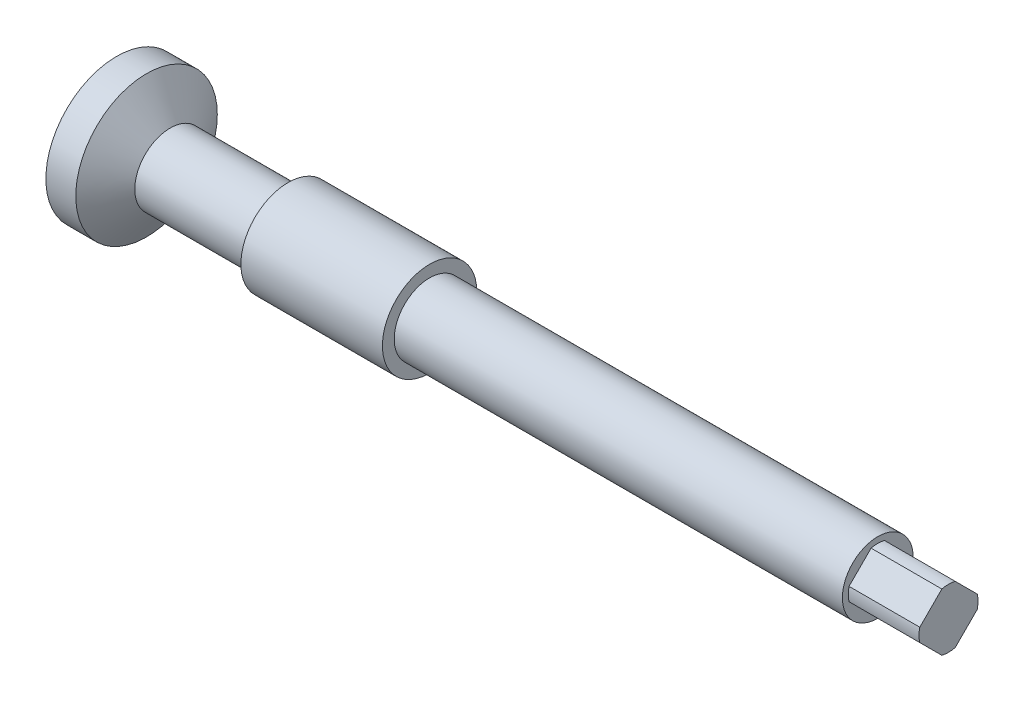
ISO-10303-21;
HEADER;
FILE_DESCRIPTION(('STEP AP214'),'2;1');
FILE_NAME('part.step','',(''),(''),'','','');
FILE_SCHEMA(('AUTOMOTIVE_DESIGN { 1 0 10303 214 1 1 1 1 }'));
ENDSEC;
DATA;
#1=APPLICATION_CONTEXT('core data for automotive mechanical design processes');
#2=APPLICATION_PROTOCOL_DEFINITION('international standard','automotive_design',2000,#1);
#3=PRODUCT_CONTEXT('',#1,'mechanical');
#4=PRODUCT('Part','Part','',(#3));
#5=PRODUCT_RELATED_PRODUCT_CATEGORY('part','',(#4));
#6=PRODUCT_DEFINITION_FORMATION('','',#4);
#7=PRODUCT_DEFINITION_CONTEXT('part definition',#1,'design');
#8=PRODUCT_DEFINITION('design','',#6,#7);
#9=PRODUCT_DEFINITION_SHAPE('','',#8);
#10=(LENGTH_UNIT() NAMED_UNIT(*) SI_UNIT(.MILLI.,.METRE.));
#11=(NAMED_UNIT(*) PLANE_ANGLE_UNIT() SI_UNIT($,.RADIAN.));
#12=(NAMED_UNIT(*) SI_UNIT($,.STERADIAN.) SOLID_ANGLE_UNIT());
#13=UNCERTAINTY_MEASURE_WITH_UNIT(LENGTH_MEASURE(1.E-05),#10,'distance_accuracy_value','');
#14=(GEOMETRIC_REPRESENTATION_CONTEXT(3) GLOBAL_UNCERTAINTY_ASSIGNED_CONTEXT((#13)) GLOBAL_UNIT_ASSIGNED_CONTEXT((#10,
#11,#12)) REPRESENTATION_CONTEXT('',''));
#15=CARTESIAN_POINT('',(0.,0.,0.));
#16=DIRECTION('',(0.,0.,1.));
#17=DIRECTION('',(1.,0.,0.));
#18=AXIS2_PLACEMENT_3D('',#15,#16,#17);
#19=CARTESIAN_POINT('',(0.,0.,0.));
#20=DIRECTION('',(1.,0.,0.));
#21=DIRECTION('',(0.,0.,-1.));
#22=AXIS2_PLACEMENT_3D('',#19,#20,#21);
#23=PLANE('',#22);
#24=CARTESIAN_POINT('',(0.,0.,0.));
#25=DIRECTION('',(1.,0.,0.));
#26=DIRECTION('',(0.,0.,-1.));
#27=AXIS2_PLACEMENT_3D('',#24,#25,#26);
#28=CIRCLE('',#27,2.5);
#29=CARTESIAN_POINT('',(0.,-0.564585653306514,-2.43541434669349));
#30=VERTEX_POINT('',#29);
#31=CARTESIAN_POINT('',(0.,0.564585653306516,-2.43541434669349));
#32=VERTEX_POINT('',#31);
#33=EDGE_CURVE('E12',#30,#32,#28,.T.);
#34=ORIENTED_EDGE('',*,*,#33,.T.);
#35=DIRECTION('',(0.,0.707106781186548,0.707106781186548));
#36=VECTOR('',#35,1.);
#37=CARTESIAN_POINT('',(0.,0.5,-2.5));
#38=LINE('',#37,#36);
#39=CARTESIAN_POINT('',(0.,2.43541434669349,-0.564585653306515));
#40=VERTEX_POINT('',#39);
#41=EDGE_CURVE('E117',#32,#40,#38,.T.);
#42=ORIENTED_EDGE('',*,*,#41,.T.);
#43=CARTESIAN_POINT('',(0.,2.43541434669349,0.564585653306515));
#44=VERTEX_POINT('',#43);
#45=EDGE_CURVE('E51',#40,#44,#28,.T.);
#46=ORIENTED_EDGE('',*,*,#45,.T.);
#47=DIRECTION('',(0.,-0.707106781186548,0.707106781186547));
#48=VECTOR('',#47,1.);
#49=CARTESIAN_POINT('',(0.,2.5,0.5));
#50=LINE('',#49,#48);
#51=CARTESIAN_POINT('',(0.,0.564585653306515,2.43541434669349));
#52=VERTEX_POINT('',#51);
#53=EDGE_CURVE('E194',#44,#52,#50,.T.);
#54=ORIENTED_EDGE('',*,*,#53,.T.);
#55=CARTESIAN_POINT('',(0.,-0.564585653306515,2.43541434669349));
#56=VERTEX_POINT('',#55);
#57=EDGE_CURVE('E63',#52,#56,#28,.T.);
#58=ORIENTED_EDGE('',*,*,#57,.T.);
#59=DIRECTION('',(0.,-0.707106781186548,-0.707106781186548));
#60=VECTOR('',#59,1.);
#61=CARTESIAN_POINT('',(0.,-2.5,0.5));
#62=LINE('',#61,#60);
#63=CARTESIAN_POINT('',(0.,-2.43541434669349,0.564585653306515));
#64=VERTEX_POINT('',#63);
#65=EDGE_CURVE('E189',#56,#64,#62,.T.);
#66=ORIENTED_EDGE('',*,*,#65,.T.);
#67=CARTESIAN_POINT('',(0.,-2.43541434669349,-0.564585653306514));
#68=VERTEX_POINT('',#67);
#69=EDGE_CURVE('E55',#64,#68,#28,.T.);
#70=ORIENTED_EDGE('',*,*,#69,.T.);
#71=DIRECTION('',(0.,0.707106781186548,-0.707106781186548));
#72=VECTOR('',#71,1.);
#73=CARTESIAN_POINT('',(0.,-0.5,-2.5));
#74=LINE('',#73,#72);
#75=EDGE_CURVE('E187',#68,#30,#74,.T.);
#76=ORIENTED_EDGE('',*,*,#75,.T.);
#77=EDGE_LOOP('',(#34,#42,#46,#54,#58,#66,#70,#76));
#78=FACE_BOUND('',#77,.T.);
#79=ADVANCED_FACE('F42',(#78),#23,.T.);
#80=CARTESIAN_POINT('',(0.,0.,0.));
#81=DIRECTION('',(1.,0.,0.));
#82=DIRECTION('',(0.,0.,-1.));
#83=AXIS2_PLACEMENT_3D('',#80,#81,#82);
#84=CYLINDRICAL_SURFACE('',#83,2.5);
#85=CARTESIAN_POINT('',(-6.,0.,0.));
#86=DIRECTION('',(1.,0.,0.));
#87=DIRECTION('',(0.,0.,-1.));
#88=AXIS2_PLACEMENT_3D('',#85,#86,#87);
#89=CIRCLE('',#88,2.5);
#90=CARTESIAN_POINT('',(-6.,2.43541434669349,-0.564585653306515));
#91=VERTEX_POINT('',#90);
#92=CARTESIAN_POINT('',(-6.,2.43541434669348,0.564585653306516));
#93=VERTEX_POINT('',#92);
#94=EDGE_CURVE('E135',#91,#93,#89,.T.);
#95=ORIENTED_EDGE('',*,*,#94,.T.);
#96=DIRECTION('',(1.,0.,0.));
#97=VECTOR('',#96,1.);
#98=CARTESIAN_POINT('',(0.,2.43541434669349,0.564585653306515));
#99=LINE('',#98,#97);
#100=EDGE_CURVE('E132',#93,#44,#99,.T.);
#101=ORIENTED_EDGE('',*,*,#100,.T.);
#102=ORIENTED_EDGE('',*,*,#45,.F.);
#103=DIRECTION('',(1.,0.,0.));
#104=VECTOR('',#103,1.);
#105=CARTESIAN_POINT('',(0.,2.43541434669348,-0.564585653306515));
#106=LINE('',#105,#104);
#107=EDGE_CURVE('E123',#40,#91,#106,.F.);
#108=ORIENTED_EDGE('',*,*,#107,.T.);
#109=EDGE_LOOP('',(#95,#101,#102,#108));
#110=FACE_BOUND('',#109,.T.);
#111=ADVANCED_FACE('F213',(#110),#84,.T.);
#112=DIRECTION('',(1.,0.,0.));
#113=VECTOR('',#112,1.);
#114=CARTESIAN_POINT('',(0.,-0.564585653306514,-2.43541434669349));
#115=LINE('',#114,#113);
#116=CARTESIAN_POINT('',(-6.,-0.564585653306515,-2.43541434669348));
#117=VERTEX_POINT('',#116);
#118=EDGE_CURVE('E124',#30,#117,#115,.F.);
#119=ORIENTED_EDGE('',*,*,#118,.T.);
#120=CARTESIAN_POINT('',(-6.,0.564585653306516,-2.43541434669348));
#121=VERTEX_POINT('',#120);
#122=EDGE_CURVE('E128',#117,#121,#89,.T.);
#123=ORIENTED_EDGE('',*,*,#122,.T.);
#124=DIRECTION('',(1.,0.,0.));
#125=VECTOR('',#124,1.);
#126=CARTESIAN_POINT('',(0.,0.564585653306516,-2.43541434669348));
#127=LINE('',#126,#125);
#128=EDGE_CURVE('E115',#121,#32,#127,.T.);
#129=ORIENTED_EDGE('',*,*,#128,.T.);
#130=ORIENTED_EDGE('',*,*,#33,.F.);
#131=EDGE_LOOP('',(#119,#123,#129,#130));
#132=FACE_BOUND('',#131,.T.);
#133=ADVANCED_FACE('F139',(#132),#84,.T.);
#134=CARTESIAN_POINT('',(-6.,-2.43541434669348,0.564585653306515));
#135=VERTEX_POINT('',#134);
#136=CARTESIAN_POINT('',(-6.,-2.43541434669348,-0.564585653306515));
#137=VERTEX_POINT('',#136);
#138=EDGE_CURVE('E140',#135,#137,#89,.T.);
#139=ORIENTED_EDGE('',*,*,#138,.T.);
#140=DIRECTION('',(1.,0.,0.));
#141=VECTOR('',#140,1.);
#142=CARTESIAN_POINT('',(0.,-2.43541434669349,-0.564585653306514));
#143=LINE('',#142,#141);
#144=EDGE_CURVE('E173',#137,#68,#143,.T.);
#145=ORIENTED_EDGE('',*,*,#144,.T.);
#146=ORIENTED_EDGE('',*,*,#69,.F.);
#147=DIRECTION('',(1.,0.,0.));
#148=VECTOR('',#147,1.);
#149=CARTESIAN_POINT('',(0.,-2.43541434669349,0.564585653306515));
#150=LINE('',#149,#148);
#151=EDGE_CURVE('E178',#64,#135,#150,.F.);
#152=ORIENTED_EDGE('',*,*,#151,.T.);
#153=EDGE_LOOP('',(#139,#145,#146,#152));
#154=FACE_BOUND('',#153,.T.);
#155=ADVANCED_FACE('F208',(#154),#84,.T.);
#156=CARTESIAN_POINT('',(-6.,0.564585653306515,2.43541434669348));
#157=VERTEX_POINT('',#156);
#158=CARTESIAN_POINT('',(-6.,-0.564585653306515,2.43541434669349));
#159=VERTEX_POINT('',#158);
#160=EDGE_CURVE('E136',#157,#159,#89,.T.);
#161=ORIENTED_EDGE('',*,*,#160,.T.);
#162=DIRECTION('',(1.,0.,0.));
#163=VECTOR('',#162,1.);
#164=CARTESIAN_POINT('',(0.,-0.564585653306515,2.43541434669349));
#165=LINE('',#164,#163);
#166=EDGE_CURVE('E177',#159,#56,#165,.T.);
#167=ORIENTED_EDGE('',*,*,#166,.T.);
#168=ORIENTED_EDGE('',*,*,#57,.F.);
#169=DIRECTION('',(1.,0.,0.));
#170=VECTOR('',#169,1.);
#171=CARTESIAN_POINT('',(0.,0.564585653306515,2.43541434669349));
#172=LINE('',#171,#170);
#173=EDGE_CURVE('E182',#52,#157,#172,.F.);
#174=ORIENTED_EDGE('',*,*,#173,.T.);
#175=EDGE_LOOP('',(#161,#167,#168,#174));
#176=FACE_BOUND('',#175,.T.);
#177=ADVANCED_FACE('F201',(#176),#84,.T.);
#178=CARTESIAN_POINT('',(-6.,2.5,0.));
#179=DIRECTION('',(1.,0.,0.));
#180=DIRECTION('',(0.,0.,-1.));
#181=AXIS2_PLACEMENT_3D('',#178,#179,#180);
#182=PLANE('',#181);
#183=DIRECTION('',(0.,-0.707106781186548,0.707106781186547));
#184=VECTOR('',#183,1.);
#185=CARTESIAN_POINT('',(-6.,2.5,0.5));
#186=LINE('',#185,#184);
#187=EDGE_CURVE('E190',#93,#157,#186,.T.);
#188=ORIENTED_EDGE('',*,*,#187,.F.);
#189=ORIENTED_EDGE('',*,*,#94,.F.);
#190=DIRECTION('',(0.,0.707106781186548,0.707106781186548));
#191=VECTOR('',#190,1.);
#192=CARTESIAN_POINT('',(-6.,0.5,-2.5));
#193=LINE('',#192,#191);
#194=EDGE_CURVE('E113',#121,#91,#193,.T.);
#195=ORIENTED_EDGE('',*,*,#194,.F.);
#196=ORIENTED_EDGE('',*,*,#122,.F.);
#197=DIRECTION('',(0.,0.707106781186548,-0.707106781186548));
#198=VECTOR('',#197,1.);
#199=CARTESIAN_POINT('',(-6.,-0.5,-2.5));
#200=LINE('',#199,#198);
#201=EDGE_CURVE('E133',#137,#117,#200,.T.);
#202=ORIENTED_EDGE('',*,*,#201,.F.);
#203=ORIENTED_EDGE('',*,*,#138,.F.);
#204=DIRECTION('',(0.,-0.707106781186548,-0.707106781186548));
#205=VECTOR('',#204,1.);
#206=CARTESIAN_POINT('',(-6.,-2.5,0.5));
#207=LINE('',#206,#205);
#208=EDGE_CURVE('E191',#159,#135,#207,.T.);
#209=ORIENTED_EDGE('',*,*,#208,.F.);
#210=ORIENTED_EDGE('',*,*,#160,.F.);
#211=EDGE_LOOP('',(#188,#189,#195,#196,#202,#203,#209,#210));
#212=FACE_BOUND('',#211,.T.);
#213=CARTESIAN_POINT('',(-6.,0.,0.));
#214=DIRECTION('',(1.,0.,0.));
#215=DIRECTION('',(0.,0.,-1.));
#216=AXIS2_PLACEMENT_3D('',#213,#214,#215);
#217=CIRCLE('',#216,3.);
#218=CARTESIAN_POINT('',(-6.,0.,-3.));
#219=VERTEX_POINT('',#218);
#220=EDGE_CURVE('E142',#219,#219,#217,.T.);
#221=ORIENTED_EDGE('',*,*,#220,.T.);
#222=EDGE_LOOP('',(#221));
#223=FACE_BOUND('',#222,.T.);
#224=ADVANCED_FACE('F130',(#212,#223),#182,.T.);
#225=CARTESIAN_POINT('',(0.,0.,0.));
#226=DIRECTION('',(1.,0.,0.));
#227=DIRECTION('',(0.,0.,-1.));
#228=AXIS2_PLACEMENT_3D('',#225,#226,#227);
#229=CYLINDRICAL_SURFACE('',#228,3.);
#230=CARTESIAN_POINT('',(-44.,0.,0.));
#231=DIRECTION('',(1.,0.,0.));
#232=DIRECTION('',(0.,0.,-1.));
#233=AXIS2_PLACEMENT_3D('',#230,#231,#232);
#234=CIRCLE('',#233,2.99999999999999);
#235=CARTESIAN_POINT('',(-44.,0.,-2.99999999999999));
#236=VERTEX_POINT('',#235);
#237=EDGE_CURVE('E149',#236,#236,#234,.T.);
#238=ORIENTED_EDGE('',*,*,#237,.T.);
#239=EDGE_LOOP('',(#238));
#240=FACE_BOUND('',#239,.T.);
#241=ORIENTED_EDGE('',*,*,#220,.F.);
#242=EDGE_LOOP('',(#241));
#243=FACE_BOUND('',#242,.T.);
#244=ADVANCED_FACE('F223',(#240,#243),#229,.T.);
#245=CARTESIAN_POINT('',(-44.,2.99999999999999,0.));
#246=DIRECTION('',(1.,0.,0.));
#247=DIRECTION('',(0.,0.,-1.));
#248=AXIS2_PLACEMENT_3D('',#245,#246,#247);
#249=PLANE('',#248);
#250=CARTESIAN_POINT('',(-44.,0.,0.));
#251=DIRECTION('',(1.,0.,0.));
#252=DIRECTION('',(0.,0.,-1.));
#253=AXIS2_PLACEMENT_3D('',#250,#251,#252);
#254=CIRCLE('',#253,3.99999999999999);
#255=CARTESIAN_POINT('',(-44.,0.,-3.99999999999999));
#256=VERTEX_POINT('',#255);
#257=EDGE_CURVE('E155',#256,#256,#254,.T.);
#258=ORIENTED_EDGE('',*,*,#257,.T.);
#259=EDGE_LOOP('',(#258));
#260=FACE_BOUND('',#259,.T.);
#261=ORIENTED_EDGE('',*,*,#237,.F.);
#262=EDGE_LOOP('',(#261));
#263=FACE_BOUND('',#262,.T.);
#264=ADVANCED_FACE('F291',(#260,#263),#249,.T.);
#265=CARTESIAN_POINT('',(0.,0.,0.));
#266=DIRECTION('',(1.,0.,0.));
#267=DIRECTION('',(0.,0.,-1.));
#268=AXIS2_PLACEMENT_3D('',#265,#266,#267);
#269=CYLINDRICAL_SURFACE('',#268,3.99999999999999);
#270=CARTESIAN_POINT('',(-56.,0.,0.));
#271=DIRECTION('',(1.,0.,0.));
#272=DIRECTION('',(0.,0.,-1.));
#273=AXIS2_PLACEMENT_3D('',#270,#271,#272);
#274=CIRCLE('',#273,3.99999999999999);
#275=CARTESIAN_POINT('',(-56.,0.,-3.99999999999999));
#276=VERTEX_POINT('',#275);
#277=EDGE_CURVE('E160',#276,#276,#274,.T.);
#278=ORIENTED_EDGE('',*,*,#277,.T.);
#279=EDGE_LOOP('',(#278));
#280=FACE_BOUND('',#279,.T.);
#281=ORIENTED_EDGE('',*,*,#257,.F.);
#282=EDGE_LOOP('',(#281));
#283=FACE_BOUND('',#282,.T.);
#284=ADVANCED_FACE('F305',(#280,#283),#269,.T.);
#285=CARTESIAN_POINT('',(-56.,3.99999999999999,0.));
#286=DIRECTION('',(-1.,0.,0.));
#287=DIRECTION('',(0.,0.,1.));
#288=AXIS2_PLACEMENT_3D('',#285,#286,#287);
#289=PLANE('',#288);
#290=CARTESIAN_POINT('',(-56.,0.,0.));
#291=DIRECTION('',(1.,0.,0.));
#292=DIRECTION('',(0.,0.,-1.));
#293=AXIS2_PLACEMENT_3D('',#290,#291,#292);
#294=CIRCLE('',#293,2.99999999999999);
#295=CARTESIAN_POINT('',(-56.,0.,-2.99999999999999));
#296=VERTEX_POINT('',#295);
#297=EDGE_CURVE('E159',#296,#296,#294,.T.);
#298=ORIENTED_EDGE('',*,*,#297,.T.);
#299=EDGE_LOOP('',(#298));
#300=FACE_BOUND('',#299,.T.);
#301=ORIENTED_EDGE('',*,*,#277,.F.);
#302=EDGE_LOOP('',(#301));
#303=FACE_BOUND('',#302,.T.);
#304=ADVANCED_FACE('F312',(#300,#303),#289,.T.);
#305=CARTESIAN_POINT('',(0.,0.,0.));
#306=DIRECTION('',(1.,0.,0.));
#307=DIRECTION('',(0.,0.,-1.));
#308=AXIS2_PLACEMENT_3D('',#305,#306,#307);
#309=CYLINDRICAL_SURFACE('',#308,2.99999999999999);
#310=CARTESIAN_POINT('',(-66.,0.,0.));
#311=DIRECTION('',(1.,0.,0.));
#312=DIRECTION('',(0.,0.,-1.));
#313=AXIS2_PLACEMENT_3D('',#310,#311,#312);
#314=CIRCLE('',#313,2.99999999999999);
#315=CARTESIAN_POINT('',(-66.,0.,-2.99999999999999));
#316=VERTEX_POINT('',#315);
#317=EDGE_CURVE('E162',#316,#316,#314,.T.);
#318=ORIENTED_EDGE('',*,*,#317,.T.);
#319=EDGE_LOOP('',(#318));
#320=FACE_BOUND('',#319,.T.);
#321=ORIENTED_EDGE('',*,*,#297,.F.);
#322=EDGE_LOOP('',(#321));
#323=FACE_BOUND('',#322,.T.);
#324=ADVANCED_FACE('F326',(#320,#323),#309,.T.);
#325=CARTESIAN_POINT('',(-66.,0.,0.));
#326=DIRECTION('',(-1.,0.,0.));
#327=DIRECTION('',(0.,0.,1.));
#328=AXIS2_PLACEMENT_3D('',#325,#326,#327);
#329=CONICAL_SURFACE('',#328,2.99999999999999,0.982793723247329);
#330=CARTESIAN_POINT('',(-68.,0.,0.));
#331=DIRECTION('',(1.,0.,0.));
#332=DIRECTION('',(0.,0.,-1.));
#333=AXIS2_PLACEMENT_3D('',#330,#331,#332);
#334=CIRCLE('',#333,5.99999999999999);
#335=CARTESIAN_POINT('',(-68.,0.,-5.99999999999999));
#336=VERTEX_POINT('',#335);
#337=EDGE_CURVE('E167',#336,#336,#334,.T.);
#338=ORIENTED_EDGE('',*,*,#337,.T.);
#339=EDGE_LOOP('',(#338));
#340=FACE_BOUND('',#339,.T.);
#341=ORIENTED_EDGE('',*,*,#317,.F.);
#342=EDGE_LOOP('',(#341));
#343=FACE_BOUND('',#342,.T.);
#344=ADVANCED_FACE('F336',(#340,#343),#329,.T.);
#345=CARTESIAN_POINT('',(0.,0.,0.));
#346=DIRECTION('',(1.,0.,0.));
#347=DIRECTION('',(0.,0.,-1.));
#348=AXIS2_PLACEMENT_3D('',#345,#346,#347);
#349=CYLINDRICAL_SURFACE('',#348,5.99999999999999);
#350=CARTESIAN_POINT('',(-70.5358983848623,0.,0.));
#351=DIRECTION('',(1.,0.,0.));
#352=DIRECTION('',(0.,0.,-1.));
#353=AXIS2_PLACEMENT_3D('',#350,#351,#352);
#354=CIRCLE('',#353,5.99999999999999);
#355=CARTESIAN_POINT('',(-70.5358983848623,0.,-5.99999999999999));
#356=VERTEX_POINT('',#355);
#357=EDGE_CURVE('E166',#356,#356,#354,.T.);
#358=ORIENTED_EDGE('',*,*,#357,.T.);
#359=EDGE_LOOP('',(#358));
#360=FACE_BOUND('',#359,.T.);
#361=ORIENTED_EDGE('',*,*,#337,.F.);
#362=EDGE_LOOP('',(#361));
#363=FACE_BOUND('',#362,.T.);
#364=ADVANCED_FACE('F347',(#360,#363),#349,.T.);
#365=CARTESIAN_POINT('',(-70.5358983848623,0.,0.));
#366=DIRECTION('',(1.,0.,0.));
#367=DIRECTION('',(0.,0.,-1.));
#368=AXIS2_PLACEMENT_3D('',#365,#366,#367);
#369=CONICAL_SURFACE('',#368,5.99999999999999,1.0471975511966);
#370=CARTESIAN_POINT('',(-74.,0.,0.));
#371=VERTEX_POINT('',#370);
#372=VERTEX_LOOP('',#371);
#373=FACE_BOUND('',#372,.T.);
#374=ORIENTED_EDGE('',*,*,#357,.F.);
#375=EDGE_LOOP('',(#374));
#376=FACE_BOUND('',#375,.T.);
#377=ADVANCED_FACE('F253',(#373,#376),#369,.T.);
#378=CARTESIAN_POINT('',(-6.,2.5,0.5));
#379=DIRECTION('',(0.,0.707106781186547,0.707106781186548));
#380=DIRECTION('',(0.,-0.707106781186548,0.707106781186547));
#381=AXIS2_PLACEMENT_3D('',#378,#379,#380);
#382=PLANE('',#381);
#383=ORIENTED_EDGE('',*,*,#53,.F.);
#384=ORIENTED_EDGE('',*,*,#100,.F.);
#385=ORIENTED_EDGE('',*,*,#187,.T.);
#386=ORIENTED_EDGE('',*,*,#173,.F.);
#387=EDGE_LOOP('',(#383,#384,#385,#386));
#388=FACE_BOUND('',#387,.T.);
#389=ADVANCED_FACE('F199',(#388),#382,.T.);
#390=CARTESIAN_POINT('',(-6.,-2.5,0.5));
#391=DIRECTION('',(0.,-0.707106781186548,0.707106781186547));
#392=DIRECTION('',(0.,-0.707106781186547,-0.707106781186548));
#393=AXIS2_PLACEMENT_3D('',#390,#391,#392);
#394=PLANE('',#393);
#395=ORIENTED_EDGE('',*,*,#65,.F.);
#396=ORIENTED_EDGE('',*,*,#166,.F.);
#397=ORIENTED_EDGE('',*,*,#208,.T.);
#398=ORIENTED_EDGE('',*,*,#151,.F.);
#399=EDGE_LOOP('',(#395,#396,#397,#398));
#400=FACE_BOUND('',#399,.T.);
#401=ADVANCED_FACE('F210',(#400),#394,.T.);
#402=CARTESIAN_POINT('',(-6.,-0.5,-2.5));
#403=DIRECTION('',(0.,-0.707106781186547,-0.707106781186547));
#404=DIRECTION('',(0.,0.707106781186548,-0.707106781186548));
#405=AXIS2_PLACEMENT_3D('',#402,#403,#404);
#406=PLANE('',#405);
#407=ORIENTED_EDGE('',*,*,#75,.F.);
#408=ORIENTED_EDGE('',*,*,#144,.F.);
#409=ORIENTED_EDGE('',*,*,#201,.T.);
#410=ORIENTED_EDGE('',*,*,#118,.F.);
#411=EDGE_LOOP('',(#407,#408,#409,#410));
#412=FACE_BOUND('',#411,.T.);
#413=ADVANCED_FACE('F209',(#412),#406,.T.);
#414=CARTESIAN_POINT('',(-6.,0.5,-2.5));
#415=DIRECTION('',(0.,0.707106781186548,-0.707106781186547));
#416=DIRECTION('',(0.,0.707106781186547,0.707106781186548));
#417=AXIS2_PLACEMENT_3D('',#414,#415,#416);
#418=PLANE('',#417);
#419=ORIENTED_EDGE('',*,*,#41,.F.);
#420=ORIENTED_EDGE('',*,*,#128,.F.);
#421=ORIENTED_EDGE('',*,*,#194,.T.);
#422=ORIENTED_EDGE('',*,*,#107,.F.);
#423=EDGE_LOOP('',(#419,#420,#421,#422));
#424=FACE_BOUND('',#423,.T.);
#425=ADVANCED_FACE('F111',(#424),#418,.T.);
#426=CLOSED_SHELL('',(#79,#111,#133,#155,#177,#224,#244,#264,#284,#304,#324,#344,#364,#377,#389,
#401,#413,#425));
#427=MANIFOLD_SOLID_BREP('B2',#426);
#428=ADVANCED_BREP_SHAPE_REPRESENTATION('',(#18,#427),#14);
#429=SHAPE_DEFINITION_REPRESENTATION(#9,#428);
ENDSEC;
END-ISO-10303-21;
